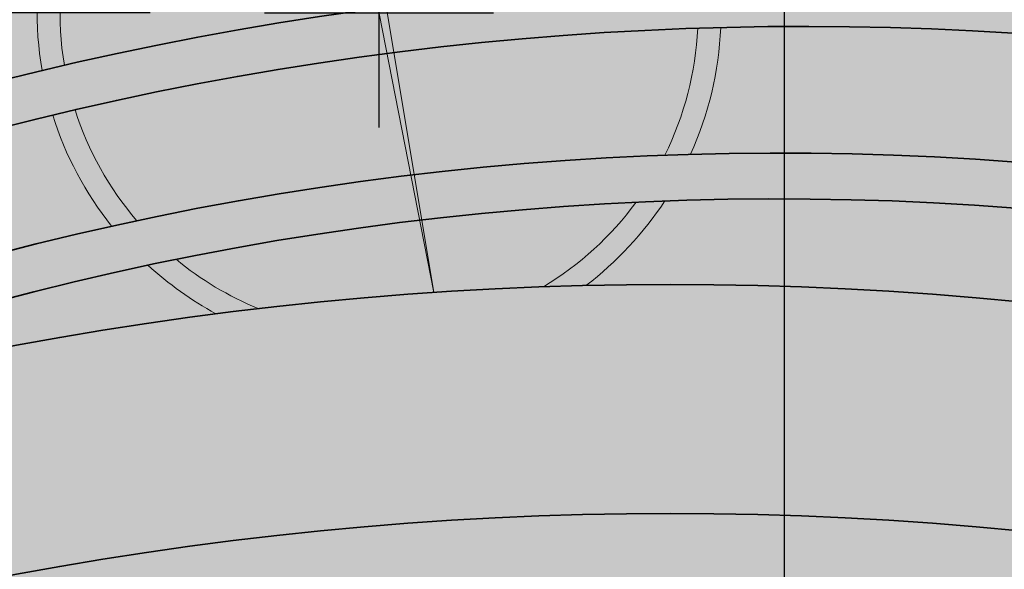
# Model space of a CAD drawing. Units: millimetres. Extents: x 130 to 1021, y 147 to 699.
# Tile 21 of 40: x 399 to 442, y 477 to 501. Entities that reach past the tile are written whole.
import ezdxf

# ---------------------------------------------------------------- set-up
doc = ezdxf.new("R2010")
doc.units = ezdxf.units.MM
doc.header["$MEASUREMENT"] = 0
for name, color, linetype, lineweight in [('A-ANNO-DIMS', 2, 'Continuous', 18), ('A-ELEV', 7, 'Continuous', 35), ('A-ELEV-PATT', 9, 'Continuous', 13), ('A-ELEV-RAIL', 6, 'Continuous', 18)]:
    doc.layers.add(name, color=color, linetype=linetype, lineweight=lineweight)
doc.styles.get("Standard").update_dxf_attribs({"font": 'arial.ttf'})
doc.dimstyles.get("Standard").update_dxf_attribs({"dimtxt": 20, "dimasz": 10, "dimexe": 10, "dimexo": 10, "dimgap": 5, "dimtad": 0, "dimtih": 1, "dimtoh": 1, "dimdec": 0, "dimzin": 0, "dimdsep": 46, "dimtxsty": 'Standard', "dimcen": 5, "dimadec": 0, "dimazin": 0, "dimtfac": 1, "dimtdec": 0, "dimtofl": 0, "dimtmove": 0, "dimatfit": 3, "dimfxl": 1, "dimtolj": 1, "dimtzin": 0, "dimarcsym": 0})

# ---------------------------------------------------------------- blocks, each defined once
blk = doc.blocks.new('*D11')
at = {"layer": 'A-ANNO-DIMS', "color": 0, "lineweight": -2, "transparency": 16777216}
for p, q in [((737.374, 648.699), (737.374, 149.739)), ((299.374, 566.947), (299.374, 149.739)), ((309.374, 159.739), (490.857, 159.739)), ((727.374, 159.739), (545.891, 159.739))]:
    blk.add_line(p, q, dxfattribs=at)
at = {"layer": 'A-ANNO-DIMS', "color": 0, "transparency": 16777216}
for points in [[(309.374, 161.406), (309.374, 158.073), (299.374, 159.739)], [(727.374, 161.406), (727.374, 158.073), (737.374, 159.739)]]:
    blk.add_solid(points, dxfattribs=at)
at = {"layer": 'Defpoints', "color": 0, "transparency": 16777216}
for p in [(737.374, 658.699), (299.374, 576.947), (737.374, 159.739)]:
    blk.add_point(p, dxfattribs=at)
at = {"layer": 'A-ANNO-DIMS', "color": 0, "transparency": 16777216, "insert": (518.374, 159.739), "char_height": 20, "attachment_point": 5}
blk.add_mtext('\\A1;438', dxfattribs=at)
blk = doc.blocks.new('*D12')
at = {"layer": 'A-ANNO-DIMS', "color": 0, "lineweight": -2, "transparency": 16777216}
for p, q in [((477.374, 661.947), (265.074, 661.947)), ((275.074, 651.947), (275.074, 438.205)), ((275.074, 194.039), (275.074, 407.782)), ((357.163, 184.039), (265.074, 184.039))]:
    blk.add_line(p, q, dxfattribs=at)
at = {"layer": 'A-ANNO-DIMS', "color": 0, "transparency": 16777216}
for points in [[(273.407, 651.947), (276.74, 651.947), (275.074, 661.947)], [(273.407, 194.039), (276.74, 194.039), (275.074, 184.039)]]:
    blk.add_solid(points, dxfattribs=at)
at = {"layer": 'Defpoints', "color": 0, "transparency": 16777216}
for p in [(275.074, 661.947), (487.374, 661.947), (367.163, 184.039)]:
    blk.add_point(p, dxfattribs=at)
at = {"layer": 'A-ANNO-DIMS', "color": 0, "transparency": 16777216, "insert": (275.074, 422.993), "char_height": 20, "attachment_point": 5}
blk.add_mtext('\\A1;477.9', dxfattribs=at)
blk = doc.blocks.new('*D15')
at = {"layer": 'A-ANNO-DIMS', "color": 0, "lineweight": -2, "transparency": 16777216}
for p, q in [((327.374, 579.884), (327.374, 696.247)), ((357.941, 411.947), (357.941, 696.247)), ((337.374, 686.247), (347.941, 686.247)), ((357.941, 686.247), (367.941, 686.247))]:
    blk.add_line(p, q, dxfattribs=at)
at = {"layer": 'A-ANNO-DIMS', "color": 0, "transparency": 16777216}
for points in [[(337.374, 687.914), (337.374, 684.581), (327.374, 686.247)], [(347.941, 687.914), (347.941, 684.581), (357.941, 686.247)]]:
    blk.add_solid(points, dxfattribs=at)
at = {"layer": 'Defpoints', "color": 0, "transparency": 16777216}
for p in [(357.941, 686.247), (327.374, 569.884), (357.941, 401.947)]:
    blk.add_point(p, dxfattribs=at)
at = {"layer": 'A-ANNO-DIMS', "color": 0, "transparency": 16777216, "insert": (406.679, 686.247), "char_height": 20, "attachment_point": 5}
blk.add_mtext('\\A1;30.57', dxfattribs=at)
blk = doc.blocks.new('*D16')
at = {"layer": 'A-ANNO-DIMS', "color": 0, "lineweight": -2, "transparency": 16777216}
for p, q in [((357.941, 411.947), (357.941, 696.247)), ((363.922, 579.884), (363.922, 696.247)), ((347.941, 686.247), (337.941, 686.247)), ((373.922, 686.247), (383.922, 686.247))]:
    blk.add_line(p, q, dxfattribs=at)
at = {"layer": 'A-ANNO-DIMS', "color": 0, "transparency": 16777216}
for points in [[(347.941, 687.914), (347.941, 684.581), (357.941, 686.247)], [(373.922, 687.914), (373.922, 684.581), (363.922, 686.247)]]:
    blk.add_solid(points, dxfattribs=at)
at = {"layer": 'Defpoints', "color": 0, "transparency": 16777216}
for p in [(363.922, 686.247), (363.922, 569.884), (357.941, 401.947)]:
    blk.add_point(p, dxfattribs=at)
at = {"layer": 'A-ANNO-DIMS', "color": 0, "transparency": 16777216, "insert": (420.737, 686.247), "char_height": 20, "attachment_point": 5}
blk.add_mtext('\\A1;5.981', dxfattribs=at)
blk = doc.blocks.new('*D17')
at = {"layer": 'A-ANNO-DIMS', "color": 0, "lineweight": -2, "transparency": 16777216}
for p, q in [((363.922, 579.884), (363.922, 696.247)), ((375.85, 490.216), (375.85, 696.247)), ((353.922, 686.247), (343.922, 686.247)), ((385.85, 686.247), (395.85, 686.247))]:
    blk.add_line(p, q, dxfattribs=at)
at = {"layer": 'A-ANNO-DIMS', "color": 0, "transparency": 16777216}
for points in [[(353.922, 687.914), (353.922, 684.581), (363.922, 686.247)], [(385.85, 687.914), (385.85, 684.581), (375.85, 686.247)]]:
    blk.add_solid(points, dxfattribs=at)
at = {"layer": 'Defpoints', "color": 0, "transparency": 16777216}
for p in [(375.85, 686.247), (363.922, 569.884), (375.85, 480.216)]:
    blk.add_point(p, dxfattribs=at)
at = {"layer": 'A-ANNO-DIMS', "color": 0, "transparency": 16777216, "insert": (441.444, 686.247), "char_height": 20, "attachment_point": 5}
blk.add_mtext('\\A1;11.928', dxfattribs=at)
blk = doc.blocks.new('*D18')
at = {"layer": 'A-ANNO-DIMS', "color": 0, "lineweight": -2, "transparency": 16777216}
for p, q in [((375.85, 490.216), (375.85, 696.247)), ((382.374, 388.947), (382.374, 696.247)), ((365.85, 686.247), (355.85, 686.247)), ((392.374, 686.247), (402.374, 686.247))]:
    blk.add_line(p, q, dxfattribs=at)
at = {"layer": 'A-ANNO-DIMS', "color": 0, "transparency": 16777216}
for points in [[(365.85, 687.914), (365.85, 684.581), (375.85, 686.247)], [(392.374, 687.914), (392.374, 684.581), (382.374, 686.247)]]:
    blk.add_solid(points, dxfattribs=at)
at = {"layer": 'Defpoints', "color": 0, "transparency": 16777216}
for p in [(382.374, 686.247), (375.85, 480.216), (382.374, 378.947)]:
    blk.add_point(p, dxfattribs=at)
at = {"layer": 'A-ANNO-DIMS', "color": 0, "transparency": 16777216, "insert": (441.132, 686.247), "char_height": 20, "attachment_point": 5}
blk.add_mtext('\\A1;6.524', dxfattribs=at)
blk = doc.blocks.new('*D19')
at = {"layer": 'A-ANNO-DIMS', "color": 0, "lineweight": -2, "transparency": 16777216}
for p, q in [((382.374, 388.947), (382.374, 696.247)), ((414.652, 510.881), (414.652, 696.247)), ((392.374, 686.247), (404.652, 686.247)), ((414.652, 686.247), (424.652, 686.247))]:
    blk.add_line(p, q, dxfattribs=at)
at = {"layer": 'A-ANNO-DIMS', "color": 0, "transparency": 16777216}
for points in [[(392.374, 687.914), (392.374, 684.581), (382.374, 686.247)], [(404.652, 687.914), (404.652, 684.581), (414.652, 686.247)]]:
    blk.add_solid(points, dxfattribs=at)
at = {"layer": 'Defpoints', "color": 0, "transparency": 16777216}
for p in [(414.652, 686.247), (414.652, 500.881), (382.374, 378.947)]:
    blk.add_point(p, dxfattribs=at)
at = {"layer": 'A-ANNO-DIMS', "color": 0, "transparency": 16777216, "insert": (463.411, 686.247), "char_height": 20, "attachment_point": 5}
blk.add_mtext('\\A1;32.28', dxfattribs=at)
blk = doc.blocks.new('*D20')
at = {"layer": 'A-ANNO-DIMS', "color": 0, "lineweight": -2, "transparency": 16777216}
for p, q in [((414.652, 510.881), (414.652, 696.247)), ((432.374, 388.947), (432.374, 696.247)), ((404.652, 686.247), (394.652, 686.247)), ((442.374, 686.247), (452.374, 686.247))]:
    blk.add_line(p, q, dxfattribs=at)
at = {"layer": 'A-ANNO-DIMS', "color": 0, "transparency": 16777216}
for points in [[(404.652, 687.914), (404.652, 684.581), (414.652, 686.247)], [(442.374, 687.914), (442.374, 684.581), (432.374, 686.247)]]:
    blk.add_solid(points, dxfattribs=at)
at = {"layer": 'Defpoints', "color": 0, "transparency": 16777216}
for p in [(432.374, 686.247), (414.652, 500.881), (432.374, 378.947)]:
    blk.add_point(p, dxfattribs=at)
at = {"layer": 'A-ANNO-DIMS', "color": 0, "transparency": 16777216, "insert": (490.075, 686.247), "char_height": 20, "attachment_point": 5}
blk.add_mtext('\\A1;17.72', dxfattribs=at)
blk = doc.blocks.new('*D21')
at = {"layer": 'A-ANNO-DIMS', "color": 0, "lineweight": -2, "transparency": 16777216}
for p, q in [((432.374, 388.947), (432.374, 696.247)), ((447.374, 656.947), (447.374, 696.247)), ((422.374, 686.247), (412.374, 686.247)), ((457.374, 686.247), (467.374, 686.247))]:
    blk.add_line(p, q, dxfattribs=at)
at = {"layer": 'A-ANNO-DIMS', "color": 0, "transparency": 16777216}
for points in [[(422.374, 687.914), (422.374, 684.581), (432.374, 686.247)], [(457.374, 687.914), (457.374, 684.581), (447.374, 686.247)]]:
    blk.add_solid(points, dxfattribs=at)
at = {"layer": 'Defpoints', "color": 0, "transparency": 16777216}
for p in [(447.374, 686.247), (447.374, 646.947), (432.374, 378.947)]:
    blk.add_point(p, dxfattribs=at)
at = {"layer": 'A-ANNO-DIMS', "color": 0, "transparency": 16777216, "insert": (485.832, 686.247), "char_height": 20, "attachment_point": 5}
blk.add_mtext('\\A1;15', dxfattribs=at)
blk = doc.blocks.new('*D22')
at = {"layer": 'A-ANNO-DIMS', "color": 0, "lineweight": -2, "transparency": 16777216}
for p, q in [((447.374, 656.947), (447.374, 696.247)), ((466.767, 403.947), (466.767, 696.247)), ((437.374, 686.247), (427.374, 686.247)), ((476.767, 686.247), (486.767, 686.247))]:
    blk.add_line(p, q, dxfattribs=at)
at = {"layer": 'A-ANNO-DIMS', "color": 0, "transparency": 16777216}
for points in [[(437.374, 687.914), (437.374, 684.581), (447.374, 686.247)], [(476.767, 687.914), (476.767, 684.581), (466.767, 686.247)]]:
    blk.add_solid(points, dxfattribs=at)
at = {"layer": 'Defpoints', "color": 0, "transparency": 16777216}
for p in [(466.767, 686.247), (447.374, 646.947), (466.767, 393.947)]:
    blk.add_point(p, dxfattribs=at)
at = {"layer": 'A-ANNO-DIMS', "color": 0, "transparency": 16777216, "insert": (532.34, 686.247), "char_height": 20, "attachment_point": 5}
blk.add_mtext('\\A1;19.393', dxfattribs=at)
blk = doc.blocks.new('*D43')
at = {"layer": 'A-ANNO-DIMS', "color": 0, "lineweight": -2, "transparency": 16777216}
for p, q in [((275.074, 510.881), (275.074, 520.881)), ((275.074, 520.881), (285.074, 520.881)), ((404.652, 500.881), (265.074, 500.881)), ((317.374, 480.95), (265.074, 480.95)), ((275.074, 470.95), (275.074, 460.95))]:
    blk.add_line(p, q, dxfattribs=at)
at = {"layer": 'A-ANNO-DIMS', "color": 0, "transparency": 16777216}
for points in [[(273.407, 510.881), (276.74, 510.881), (275.074, 500.881)], [(273.407, 470.95), (276.74, 470.95), (275.074, 480.95)]]:
    blk.add_solid(points, dxfattribs=at)
at = {"layer": 'Defpoints', "color": 0, "transparency": 16777216}
for p in [(275.074, 500.881), (414.652, 500.881), (327.374, 480.95)]:
    blk.add_point(p, dxfattribs=at)
at = {"layer": 'A-ANNO-DIMS', "color": 0, "transparency": 16777216, "insert": (322.877, 520.881), "char_height": 20, "attachment_point": 5}
blk.add_mtext('\\A1;19.93', dxfattribs=at)
blk = doc.blocks.new('*D62')
at = {"layer": 'A-ANNO-DIMS', "color": 0, "lineweight": -2, "transparency": 16777216}
for p, q in [((414.652, 495.881), (414.652, 505.881)), ((379.725, 501.926), (389.721, 501.627)), ((409.652, 500.881), (419.652, 500.881))]:
    blk.add_line(p, q, dxfattribs=at)
at = {"layer": 'A-ANNO-DIMS', "color": 0, "transparency": 16777216}
blk.add_solid([(389.771, 503.293), (389.671, 499.961), (399.716, 501.328)], dxfattribs=at)
at = {"layer": 'Defpoints', "color": 0, "transparency": 16777216}
for p in [(399.716, 501.328), (429.589, 500.434)]:
    blk.add_point(p, dxfattribs=at)
at = {"layer": 'A-ANNO-DIMS', "color": 0, "transparency": 16777216, "insert": (322.338, 501.926), "char_height": 20, "attachment_point": 5}
blk.add_mtext('\\A1;∅29.886', dxfattribs=at)
blk = doc.blocks.new('*D63')
at = {"layer": 'A-ANNO-DIMS', "color": 0, "lineweight": -2, "transparency": 16777216}
for p, q in [((414.652, 495.881), (414.652, 505.881)), ((380.753, 502.59), (390.74, 502.086)), ((409.652, 500.881), (419.652, 500.881))]:
    blk.add_line(p, q, dxfattribs=at)
at = {"layer": 'A-ANNO-DIMS', "color": 0, "transparency": 16777216}
blk.add_solid([(390.824, 503.751), (390.656, 500.422), (400.727, 501.583)], dxfattribs=at)
at = {"layer": 'Defpoints', "color": 0, "transparency": 16777216}
for p in [(400.727, 501.583), (428.578, 500.179)]:
    blk.add_point(p, dxfattribs=at)
at = {"layer": 'A-ANNO-DIMS', "color": 0, "transparency": 16777216, "insert": (323.365, 502.59), "char_height": 20, "attachment_point": 5}
blk.add_mtext('\\A1;∅27.886', dxfattribs=at)
blk = doc.blocks.new('*D65')
at = {"layer": 'A-ANNO-DIMS', "color": 0, "lineweight": -2, "transparency": 16777216}
for p, q in [((495.463, 509.127), (472.508, 423.108)), ((505.463, 509.127), (495.463, 509.127)), ((427.374, 248.979), (427.374, 258.979)), ((422.374, 253.979), (432.374, 253.979))]:
    blk.add_line(p, q, dxfattribs=at)
at = {"layer": 'A-ANNO-DIMS', "color": 0, "transparency": 16777216}
blk.add_solid([(470.898, 423.538), (474.118, 422.679), (469.93, 413.447)], dxfattribs=at)
at = {"layer": 'Defpoints', "color": 0, "transparency": 16777216}
for p in [(469.93, 413.447), (427.374, 253.979)]:
    blk.add_point(p, dxfattribs=at)
at = {"layer": 'A-ANNO-DIMS', "color": 0, "transparency": 16777216, "insert": (561.623, 509.127), "char_height": 20, "attachment_point": 5}
blk.add_mtext('\\A1;R165.05', dxfattribs=at)
blk = doc.blocks.new('*D66')
at = {"layer": 'A-ANNO-DIMS', "color": 0, "lineweight": -2, "transparency": 16777216}
for p, q in [((341.579, 557.194), (351.579, 557.194)), ((351.579, 557.194), (376.947, 478.135)), ((427.374, 315.978), (427.374, 325.978)), ((422.374, 320.978), (432.374, 320.978))]:
    blk.add_line(p, q, dxfattribs=at)
at = {"layer": 'A-ANNO-DIMS', "color": 0, "transparency": 16777216}
blk.add_solid([(378.534, 478.644), (375.36, 477.626), (380.002, 468.613)], dxfattribs=at)
at = {"layer": 'Defpoints', "color": 0, "transparency": 16777216}
for p in [(380.002, 468.613), (427.374, 320.978)]:
    blk.add_point(p, dxfattribs=at)
at = {"layer": 'A-ANNO-DIMS', "color": 0, "transparency": 16777216, "insert": (263.53, 557.194), "char_height": 20, "attachment_point": 5}
blk.add_mtext('\\A1;4X R155.05', dxfattribs=at)
blk = doc.blocks.new('*D67')
at = {"layer": 'A-ANNO-DIMS', "color": 0, "lineweight": -2, "transparency": 16777216}
for p, q in [((479.756, 492.431), (462.144, 412.223)), ((489.756, 492.431), (479.756, 492.431)), ((427.07, 247.496), (427.07, 257.496)), ((422.07, 252.496), (432.07, 252.496))]:
    blk.add_line(p, q, dxfattribs=at)
at = {"layer": 'A-ANNO-DIMS', "color": 0, "transparency": 16777216}
blk.add_solid([(460.516, 412.58), (463.772, 411.865), (459.999, 402.455)], dxfattribs=at)
at = {"layer": 'Defpoints', "color": 0, "transparency": 16777216}
for p in [(459.999, 402.455), (427.07, 252.496)]:
    blk.add_point(p, dxfattribs=at)
at = {"layer": 'A-ANNO-DIMS', "color": 0, "transparency": 16777216, "insert": (545.841, 492.431), "char_height": 20, "attachment_point": 5}
blk.add_mtext('\\A1;R153.53', dxfattribs=at)
blk = doc.blocks.new('*D68')
at = {"layer": 'A-ANNO-DIMS', "color": 0, "lineweight": -2, "transparency": 16777216}
for p, q in [((361.841, 579.756), (371.841, 579.756)), ((371.841, 579.756), (392.167, 506.693)), ((433.191, 354.23), (433.191, 364.23)), ((428.191, 359.23), (438.191, 359.23))]:
    blk.add_line(p, q, dxfattribs=at)
at = {"layer": 'A-ANNO-DIMS', "color": 0, "transparency": 16777216}
blk.add_solid([(393.773, 507.14), (390.561, 506.246), (394.847, 497.059)], dxfattribs=at)
at = {"layer": 'Defpoints', "color": 0, "transparency": 16777216}
for p in [(394.847, 497.059), (433.191, 359.23)]:
    blk.add_point(p, dxfattribs=at)
at = {"layer": 'A-ANNO-DIMS', "color": 0, "transparency": 16777216, "insert": (305.764, 579.756), "char_height": 20, "attachment_point": 5}
blk.add_mtext('\\A1;R143.06', dxfattribs=at)
blk = doc.blocks.new('*D69')
at = {"layer": 'A-ANNO-DIMS', "color": 0, "lineweight": -2, "transparency": 16777216}
for p, q in [((507.746, 572.261), (483.091, 501.813)), ((517.746, 572.261), (507.746, 572.261)), ((433.191, 354.23), (433.191, 364.23)), ((428.191, 359.23), (438.191, 359.23))]:
    blk.add_line(p, q, dxfattribs=at)
at = {"layer": 'A-ANNO-DIMS', "color": 0, "transparency": 16777216}
blk.add_solid([(481.518, 502.363), (484.664, 501.262), (479.788, 492.374)], dxfattribs=at)
at = {"layer": 'Defpoints', "color": 0, "transparency": 16777216}
for p in [(479.788, 492.374), (433.191, 359.23)]:
    blk.add_point(p, dxfattribs=at)
at = {"layer": 'A-ANNO-DIMS', "color": 0, "transparency": 16777216, "insert": (573.824, 572.261), "char_height": 20, "attachment_point": 5}
blk.add_mtext('\\A1;R141.06', dxfattribs=at)
blk = doc.blocks.new('*D70')
at = {"layer": 'A-ANNO-DIMS', "color": 0, "lineweight": -2, "transparency": 16777216}
for p, q in [((370.141, 588.4), (380.141, 588.4)), ((380.141, 588.4), (397.473, 517.008)), ((432.65, 367.109), (432.65, 377.109)), ((427.65, 372.109), (437.65, 372.109))]:
    blk.add_line(p, q, dxfattribs=at)
at = {"layer": 'A-ANNO-DIMS', "color": 0, "transparency": 16777216}
blk.add_solid([(399.093, 517.402), (395.854, 516.615), (399.832, 507.291)], dxfattribs=at)
at = {"layer": 'Defpoints', "color": 0, "transparency": 16777216}
for p in [(399.832, 507.291), (432.65, 372.109)]:
    blk.add_point(p, dxfattribs=at)
at = {"layer": 'A-ANNO-DIMS', "color": 0, "transparency": 16777216, "insert": (323.757, 588.4), "char_height": 20, "attachment_point": 5}
blk.add_mtext('\\A1;R139.1', dxfattribs=at)
blk = doc.blocks.new('*D71')
at = {"layer": 'A-ANNO-DIMS', "color": 0, "lineweight": -2, "transparency": 16777216}
for p, q in [((492.108, 581.609), (472.542, 512.666)), ((502.108, 581.609), (492.108, 581.609)), ((432.65, 367.109), (432.65, 377.109)), ((427.65, 372.109), (437.65, 372.109))]:
    blk.add_line(p, q, dxfattribs=at)
at = {"layer": 'A-ANNO-DIMS', "color": 0, "transparency": 16777216}
blk.add_solid([(470.938, 513.121), (474.145, 512.211), (469.812, 503.046)], dxfattribs=at)
at = {"layer": 'Defpoints', "color": 0, "transparency": 16777216}
for p in [(469.812, 503.046), (432.65, 372.109)]:
    blk.add_point(p, dxfattribs=at)
at = {"layer": 'A-ANNO-DIMS', "color": 0, "transparency": 16777216, "insert": (548.493, 581.609), "char_height": 20, "attachment_point": 5}
blk.add_mtext('\\A1;R136.1', dxfattribs=at)
blk = doc.blocks.new('*D72')
at = {"layer": 'A-ANNO-DIMS', "color": 0, "lineweight": -2, "transparency": 16777216}
for p, q in [((460.658, 573.64), (451.279, 503.49)), ((470.658, 573.64), (460.658, 573.64)), ((432.115, 355.142), (432.115, 365.142)), ((427.115, 360.142), (437.115, 360.142))]:
    blk.add_line(p, q, dxfattribs=at)
at = {"layer": 'A-ANNO-DIMS', "color": 0, "transparency": 16777216}
blk.add_solid([(449.628, 503.711), (452.931, 503.27), (449.954, 493.579)], dxfattribs=at)
at = {"layer": 'Defpoints', "color": 0, "transparency": 16777216}
for p in [(449.954, 493.579), (432.115, 360.142)]:
    blk.add_point(p, dxfattribs=at)
at = {"layer": 'A-ANNO-DIMS', "color": 0, "transparency": 16777216, "insert": (526.64, 573.64), "char_height": 20, "attachment_point": 5}
blk.add_mtext('\\A1;R134.62', dxfattribs=at)
blk = doc.blocks.new('*D73')
at = {"layer": 'A-ANNO-DIMS', "color": 0, "lineweight": -2, "transparency": 16777216}
for p, q in [((402.678, 571.448), (412.678, 571.448)), ((412.678, 571.448), (419.051, 502.166)), ((432.115, 355.142), (432.115, 365.142)), ((427.115, 360.142), (437.115, 360.142))]:
    blk.add_line(p, q, dxfattribs=at)
at = {"layer": 'A-ANNO-DIMS', "color": 0, "transparency": 16777216}
blk.add_solid([(420.711, 502.319), (417.391, 502.014), (419.967, 492.208)], dxfattribs=at)
at = {"layer": 'Defpoints', "color": 0, "transparency": 16777216}
for p in [(419.967, 492.208), (432.115, 360.142)]:
    blk.add_point(p, dxfattribs=at)
at = {"layer": 'A-ANNO-DIMS', "color": 0, "transparency": 16777216, "insert": (346.696, 571.448), "char_height": 20, "attachment_point": 5}
blk.add_mtext('\\A1;R132.62', dxfattribs=at)

msp = doc.modelspace()

# ---------------------------------------------------------------- hatches: boundary and pattern name
at = {"layer": 'A-ELEV-PATT'}
h = msp.add_hatch(color=256, dxfattribs=at)
h.dxf.hatch_style = 1
h.paths.add_polyline_path([(737.3738, 658.6988, 0.0135961), (632.4019, 661.9473), (607.3738, 661.9473), (487.3738, 661.9473), (487.3738, 649.9473), (607.3738, 649.9473), (632.3794, 649.9473, -0.0136841), (737.3738, 646.6784)])
h.paths.add_polyline_path([(732.3738, 643.9599, 0.0130529), (632.3738, 646.9473), (607.3738, 646.9473), (487.3738, 646.9473), (487.3738, 596.9473), (632.3738, 596.9473, -0.0130529), (732.3738, 593.9599)])
h.paths.add_polyline_path([(737.3738, 593.6732, 0.0137063), (632.3738, 596.9473), (487.3738, 596.9473), (487.3738, 586.9473), (632.355, 586.9473, -0.0137808), (737.3738, 583.6559)])
h.paths.add_polyline_path([(447.3738, 646.9473), (307.3738, 646.9473), (302.3738, 646.9473), (302.3738, 634.9473), (447.3738, 634.9473)])
h.paths.add_polyline_path([(447.3738, 631.9473), (307.3738, 631.9473), (307.3738, 586.9473), (447.3738, 586.9473)])
h.paths.add_polyline_path([(447.3738, 586.9473), (307.3738, 586.9473), (302.3738, 586.9473), (302.3738, 576.9473), (447.3738, 576.9473)])
h.paths.add_polyline_path([(447.3738, 573.9473), (367.3738, 573.9473), (367.3738, 539.9473), (447.3738, 539.9473)])
h.paths.add_polyline_path([(447.3738, 537.9473), (367.3738, 537.9473), (367.3738, 507.9473), (400.392, 507.4253, -0.001728), (401.3281, 507.6451, -0.5220025), (425.6117, 511.0391, -0.0391849), (447.3738, 510.4359), (447.3738, 510.7883)])
h.paths.add_polyline_path([(394.7238, 505.9473), (367.3738, 505.9473), (367.3738, 476.9473, -0.0146512), (375.8501, 480.2159), (376.1506, 499.2266, -0.0355419)])
h.paths.add_polyline_path([(632.3738, 583.9473), (552.3738, 583.9473), (552.3738, 550.9473), (632.3738, 550.9473)])
h.paths.add_polyline_path([(632.3738, 548.9473), (552.3738, 548.9473), (552.3738, 515.9473), (632.3738, 515.9473)])
h.paths.add_polyline_path([(632.3738, 513.9473), (552.3738, 513.9473), (552.3738, 476.9473), (632.3738, 476.9473)])
h.paths.add_polyline_path([(737.3738, 473.6903, 0.0136326), (632.3926, 476.9473), (552.3738, 476.9473), (487.3738, 476.9473), (487.3738, 466.9473), (632.3738, 466.9473, -0.0137063), (737.3738, 463.6732)])
h.paths.add_polyline_path([(732.3738, 460.9552, 0.0130741), (632.3681, 463.9473), (487.3738, 463.9473), (487.3738, 407.735, -0.0032286), (489.3544, 406.9473), (632.3926, 406.9473, -0.0129826), (732.3738, 403.9755)])
h.paths.add_polyline_path([(487.3738, 463.9473, 0.20133), (367.3738, 463.9473), (367.3738, 407.735, -0.1882031), (487.3738, 407.735)])
h.paths.add_polyline_path([(367.3738, 476.9473), (367.3738, 466.9473, -0.2013309), (487.3738, 466.9473), (487.3738, 476.9473, 0.20133)])
h.paths.add_polyline_path([(367.3738, 463.9473), (307.3738, 463.9473), (307.3738, 401.9473), (357.9413, 401.9473), (367.3738, 407.735)])
h.paths.add_polyline_path([(367.3738, 476.9473), (302.3738, 476.9473), (302.3738, 466.9473), (367.3738, 466.9473)])
h.paths.add_polyline_path([(632.8184, 366.9453), (552.3738, 366.9453), (552.3738, 393.9473), (632.8184, 393.9473)])
h.paths.add_polyline_path([(632.8184, 357.2114), (632.8184, 363.9453), (552.3738, 363.9453), (552.3738, 357.2114), (552.3738, 336.9453), (632.8184, 336.9453)])
h.paths.add_polyline_path([(632.8184, 333.9453), (552.3738, 333.9453), (552.3738, 306.9453), (632.8184, 306.9453)])
h.paths.add_polyline_path([(632.8184, 303.9453), (552.3738, 303.9453), (552.3738, 273.9473), (632.355, 273.9473, 0.0000608), (632.8184, 273.9491)])
h.paths.add_polyline_path([(737.3738, 403.6903, 0.0136326), (632.3926, 406.9473), (489.3544, 406.9473, 0.1915481), (367.3738, 407.735), (367.3738, 396.9473, -0.2013309), (487.3738, 396.9473), (632.3738, 396.9473, -0.0137063), (737.3738, 393.6732)])
h.paths.add_polyline_path([(357.9413, 401.9473), (307.3738, 401.9473), (307.3738, 391.9473), (357.9413, 391.9473)])
h.paths.add_polyline_path([(357.9413, 357.2114), (357.9413, 388.9473), (307.3738, 388.9473), (307.3738, 357.2114), (307.3738, 273.9473), (357.9413, 273.9473)])
h.paths.add_polyline_path([(732.3738, 263.93, -0.0130317), (632.3794, 260.9473), (466.7667, 260.9473), (466.7667, 240.9473), (469.8406, 236.978), (469.8406, 221.978), (472.9145, 218.0087), (472.9145, 213.9473), (607.3738, 213.9473), (732.3738, 213.9473)])
h.paths.add_polyline_path([(732.3738, 290.889), (722.479, 290.889), (722.479, 301.889), (732.3738, 301.889), (732.3738, 305.889), (722.479, 305.889), (722.479, 316.889), (732.3738, 316.889), (732.3738, 320.889), (722.479, 320.889), (722.479, 331.889), (732.3738, 331.889), (732.3738, 335.889), (722.479, 335.889), (722.479, 346.889), (732.3738, 346.889), (732.3738, 350.889), (722.479, 350.889), (722.479, 361.889), (732.3738, 361.889), (732.3738, 365.889), (722.479, 365.889), (722.479, 376.889), (732.3738, 376.889), (732.3738, 380.889), (722.479, 380.889), (722.479, 391.4848, 0.0005233), (718.479, 391.6843), (718.479, 380.889), (707.479, 380.889), (707.479, 392.1896, 0.0005231), (703.479, 392.3576), (703.479, 380.889), (692.479, 380.889), (692.479, 392.7765, 0.0005229), (688.479, 392.9131), (688.479, 380.889), (677.479, 380.889), (677.479, 393.2456, 0.0005228), (673.479, 393.3508), (673.479, 380.889), (662.479, 380.889), (662.479, 393.597, 0.0005227), (658.479, 393.6709), (658.479, 380.889), (647.479, 380.889), (647.479, 393.8308, 0.0005226), (643.479, 393.8732), (643.479, 380.889), (632.8184, 380.889), (632.8184, 376.889), (643.479, 376.889), (643.479, 365.889), (632.8184, 365.889), (632.8184, 361.889), (643.479, 361.889), (643.479, 350.889), (632.8184, 350.889), (632.8184, 346.889), (643.479, 346.889), (643.479, 335.889), (632.8184, 335.889), (632.8184, 331.889), (643.479, 331.889), (643.479, 320.889), (632.8184, 320.889), (632.8184, 316.889), (643.479, 316.889), (643.479, 305.889), (632.8184, 305.889), (632.8184, 301.889), (643.479, 301.889), (643.479, 290.889), (632.8184, 290.889), (632.8184, 286.889), (643.479, 286.889), (643.479, 274.0217, 0.0005246), (647.479, 274.0643), (647.479, 286.889), (658.479, 286.889), (658.479, 274.2248, 0.0005246), (662.479, 274.2989), (662.479, 286.889), (673.479, 286.889), (673.479, 274.546, 0.0005247), (677.479, 274.6516), (677.479, 286.889), (688.479, 286.889), (688.479, 274.9853, 0.0005248), (692.479, 275.1224), (692.479, 286.889), (703.479, 286.889), (703.479, 275.5429, 0.000525), (707.479, 275.7115), (707.479, 286.889), (718.479, 286.889), (718.479, 276.2187, 0.0005252), (722.479, 276.4189), (722.479, 286.889), (732.3738, 286.889)])
h.paths.add_polyline_path([(718.479, 290.889), (707.479, 290.889), (707.479, 301.889), (718.479, 301.889)], flags=16)
h.paths.add_polyline_path([(703.479, 290.889), (692.479, 290.889), (692.479, 301.889), (703.479, 301.889)], flags=16)
h.paths.add_polyline_path([(718.479, 305.889), (707.479, 305.889), (707.479, 316.889), (718.479, 316.889)], flags=16)
h.paths.add_polyline_path([(703.479, 305.889), (692.479, 305.889), (692.479, 316.889), (703.479, 316.889)], flags=16)
h.paths.add_polyline_path([(688.479, 290.889), (677.479, 290.889), (677.479, 301.889), (688.479, 301.889)], flags=16)
h.paths.add_polyline_path([(718.479, 320.889), (707.479, 320.889), (707.479, 331.889), (718.479, 331.889)], flags=16)
h.paths.add_polyline_path([(688.479, 305.889), (677.479, 305.889), (677.479, 316.889), (688.479, 316.889)], flags=16)
h.paths.add_polyline_path([(703.479, 320.889), (692.479, 320.889), (692.479, 331.889), (703.479, 331.889)], flags=16)
h.paths.add_polyline_path([(688.479, 320.889), (677.479, 320.889), (677.479, 331.889), (688.479, 331.889)], flags=16)
h.paths.add_polyline_path([(673.479, 290.889), (662.479, 290.889), (662.479, 301.889), (673.479, 301.889)], flags=16)
h.paths.add_polyline_path([(718.479, 335.889), (707.479, 335.889), (707.479, 346.889), (718.479, 346.889)], flags=16)
h.paths.add_polyline_path([(673.479, 305.889), (662.479, 305.889), (662.479, 316.889), (673.479, 316.889)], flags=16)
h.paths.add_polyline_path([(703.479, 335.889), (692.479, 335.889), (692.479, 346.889), (703.479, 346.889)], flags=16)
h.paths.add_polyline_path([(673.479, 320.889), (662.479, 320.889), (662.479, 331.889), (673.479, 331.889)], flags=16)
h.paths.add_polyline_path([(688.479, 335.889), (677.479, 335.889), (677.479, 346.889), (688.479, 346.889)], flags=16)
h.paths.add_polyline_path([(658.479, 290.889), (647.479, 290.889), (647.479, 301.889), (658.479, 301.889)], flags=16)
h.paths.add_polyline_path([(718.479, 350.889), (707.479, 350.889), (707.479, 361.889), (718.479, 361.889)], flags=16)
h.paths.add_polyline_path([(658.479, 305.889), (647.479, 305.889), (647.479, 316.889), (658.479, 316.889)], flags=16)
h.paths.add_polyline_path([(703.479, 350.889), (692.479, 350.889), (692.479, 361.889), (703.479, 361.889)], flags=16)
h.paths.add_polyline_path([(673.479, 335.889), (662.479, 335.889), (662.479, 346.889), (673.479, 346.889)], flags=16)
h.paths.add_polyline_path([(658.479, 320.889), (647.479, 320.889), (647.479, 331.889), (658.479, 331.889)], flags=16)
h.paths.add_polyline_path([(688.479, 350.889), (677.479, 350.889), (677.479, 361.889), (688.479, 361.889)], flags=16)
h.paths.add_polyline_path([(718.479, 365.889), (707.479, 365.889), (707.479, 376.889), (718.479, 376.889)], flags=16)
h.paths.add_polyline_path([(658.479, 335.889), (647.479, 335.889), (647.479, 346.889), (658.479, 346.889)], flags=16)
h.paths.add_polyline_path([(673.479, 350.889), (662.479, 350.889), (662.479, 361.889), (673.479, 361.889)], flags=16)
h.paths.add_polyline_path([(703.479, 365.889), (692.479, 365.889), (692.479, 376.889), (703.479, 376.889)], flags=16)
h.paths.add_polyline_path([(688.479, 365.889), (677.479, 365.889), (677.479, 376.889), (688.479, 376.889)], flags=16)
h.paths.add_polyline_path([(658.479, 350.889), (647.479, 350.889), (647.479, 361.889), (658.479, 361.889)], flags=16)
h.paths.add_polyline_path([(673.479, 365.889), (662.479, 365.889), (662.479, 376.889), (673.479, 376.889)], flags=16)
h.paths.add_polyline_path([(658.479, 365.889), (647.479, 365.889), (647.479, 376.889), (658.479, 376.889)], flags=16)
h.paths.add_polyline_path([(732.3738, 503.9786), (722.3392, 503.9786), (722.3392, 514.9786), (732.3738, 514.9786), (732.3738, 518.9786), (722.3392, 518.9786), (722.3392, 529.9786), (732.3738, 529.9786), (732.3738, 533.9786), (722.3392, 533.9786), (722.3392, 544.9786), (732.3738, 544.9786), (732.3738, 546.9473), (732.3738, 548.9786), (722.3392, 548.9786), (722.3392, 559.9786), (732.3738, 559.9786), (732.3738, 563.9786), (722.3392, 563.9786), (722.3392, 574.9786), (732.3738, 574.9786), (732.3738, 578.9786), (722.3392, 578.9786), (722.3392, 581.4789, 0.000526), (718.3392, 581.6791), (718.3392, 578.9786), (707.3392, 578.9786), (707.3392, 582.1863, 0.0005258), (703.3392, 582.355), (703.3392, 578.9786), (692.3392, 578.9786), (692.3392, 582.7752, 0.0005257), (688.3392, 582.9123), (688.3392, 578.9786), (677.3392, 578.9786), (677.3392, 583.2457, 0.0005255), (673.3392, 583.3512), (673.3392, 578.9786), (662.3392, 578.9786), (662.3392, 583.5978, 0.0005254), (658.3392, 583.6718), (658.3392, 578.9786), (647.3392, 578.9786), (647.3392, 583.8317, 0.0005254), (643.3392, 583.8741), (643.3392, 578.9786), (632.3738, 578.9786), (632.3738, 574.9786), (643.3392, 574.9786), (643.3392, 563.9786), (632.3738, 563.9786), (632.3738, 559.9786), (643.3392, 559.9786), (643.3392, 548.9786), (632.3738, 548.9786), (632.3738, 544.9786), (643.3392, 544.9786), (643.3392, 533.9786), (632.3738, 533.9786), (632.3738, 529.9786), (643.3392, 529.9786), (643.3392, 518.9786), (632.3738, 518.9786), (632.3738, 515.9473), (632.3738, 514.9786), (643.3392, 514.9786), (643.3392, 503.9786), (632.3738, 503.9786), (632.3738, 499.9786), (643.3392, 499.9786), (643.3392, 488.9786), (632.3738, 488.9786), (632.3738, 484.9786), (643.3392, 484.9786), (643.3392, 476.8751, -0.0005191), (647.3392, 476.8332), (647.3392, 484.9786), (658.3392, 484.9786), (658.3392, 476.6752, -0.0005192), (662.3392, 476.6022), (662.3392, 484.9786), (673.3392, 484.9786), (673.3392, 476.3585, -0.0005193), (677.3392, 476.2543), (677.3392, 484.9786), (688.3392, 484.9786), (688.3392, 475.9248, -0.0005194), (692.3392, 475.7894), (692.3392, 484.9786), (703.3392, 484.9786), (703.3392, 475.3741, -0.0005195), (707.3392, 475.2075), (707.3392, 484.9786), (718.3392, 484.9786), (718.3392, 474.7064, -0.0005197), (722.3392, 474.5086), (722.3392, 484.9786), (732.3738, 484.9786), (732.3738, 488.9786), (722.3392, 488.9786), (722.3392, 499.9786), (732.3738, 499.9786)])
h.paths.add_polyline_path([(718.3392, 503.9786), (707.3392, 503.9786), (707.3392, 514.9786), (718.3392, 514.9786)], flags=16)
h.paths.add_polyline_path([(718.3392, 499.9786), (718.3392, 488.9786), (707.3392, 488.9786), (707.3392, 499.9786)], flags=16)
h.paths.add_polyline_path([(718.3392, 518.9786), (707.3392, 518.9786), (707.3392, 529.9786), (718.3392, 529.9786)], flags=16)
h.paths.add_polyline_path([(703.3392, 503.9786), (692.3392, 503.9786), (692.3392, 514.9786), (703.3392, 514.9786)], flags=16)
h.paths.add_polyline_path([(703.3392, 499.9786), (703.3392, 488.9786), (692.3392, 488.9786), (692.3392, 499.9786)], flags=16)
h.paths.add_polyline_path([(703.3392, 518.9786), (692.3392, 518.9786), (692.3392, 529.9786), (703.3392, 529.9786)], flags=16)
h.paths.add_polyline_path([(718.3392, 533.9786), (707.3392, 533.9786), (707.3392, 544.9786), (718.3392, 544.9786)], flags=16)
h.paths.add_polyline_path([(688.3392, 503.9786), (677.3392, 503.9786), (677.3392, 514.9786), (688.3392, 514.9786)], flags=16)
h.paths.add_polyline_path([(688.3392, 499.9786), (688.3392, 488.9786), (677.3392, 488.9786), (677.3392, 499.9786)], flags=16)
h.paths.add_polyline_path([(703.3392, 533.9786), (692.3392, 533.9786), (692.3392, 544.9786), (703.3392, 544.9786)], flags=16)
h.paths.add_polyline_path([(688.3392, 518.9786), (677.3392, 518.9786), (677.3392, 529.9786), (688.3392, 529.9786)], flags=16)
h.paths.add_polyline_path([(688.3392, 533.9786), (677.3392, 533.9786), (677.3392, 544.9786), (688.3392, 544.9786)], flags=16)
h.paths.add_polyline_path([(718.3392, 548.9786), (707.3392, 548.9786), (707.3392, 559.9786), (718.3392, 559.9786)], flags=16)
h.paths.add_polyline_path([(673.3392, 503.9786), (662.3392, 503.9786), (662.3392, 514.9786), (673.3392, 514.9786)], flags=16)
h.paths.add_polyline_path([(673.3392, 499.9786), (673.3392, 488.9786), (662.3392, 488.9786), (662.3392, 499.9786)], flags=16)
h.paths.add_polyline_path([(703.3392, 548.9786), (692.3392, 548.9786), (692.3392, 559.9786), (703.3392, 559.9786)], flags=16)
h.paths.add_polyline_path([(673.3392, 518.9786), (662.3392, 518.9786), (662.3392, 529.9786), (673.3392, 529.9786)], flags=16)
h.paths.add_polyline_path([(688.3392, 548.9786), (677.3392, 548.9786), (677.3392, 559.9786), (688.3392, 559.9786)], flags=16)
h.paths.add_polyline_path([(673.3392, 533.9786), (662.3392, 533.9786), (662.3392, 544.9786), (673.3392, 544.9786)], flags=16)
h.paths.add_polyline_path([(718.3392, 563.9786), (707.3392, 563.9786), (707.3392, 574.9786), (718.3392, 574.9786)], flags=16)
h.paths.add_polyline_path([(658.3392, 503.9786), (647.3392, 503.9786), (647.3392, 514.9786), (658.3392, 514.9786)], flags=16)
h.paths.add_polyline_path([(658.3392, 499.9786), (658.3392, 488.9786), (647.3392, 488.9786), (647.3392, 499.9786)], flags=16)
h.paths.add_polyline_path([(703.3392, 563.9786), (692.3392, 563.9786), (692.3392, 574.9786), (703.3392, 574.9786)], flags=16)
h.paths.add_polyline_path([(658.3392, 518.9786), (647.3392, 518.9786), (647.3392, 529.9786), (658.3392, 529.9786)], flags=16)
h.paths.add_polyline_path([(673.3392, 548.9786), (662.3392, 548.9786), (662.3392, 559.9786), (673.3392, 559.9786)], flags=16)
h.paths.add_polyline_path([(688.3392, 563.9786), (677.3392, 563.9786), (677.3392, 574.9786), (688.3392, 574.9786)], flags=16)
h.paths.add_polyline_path([(658.3392, 533.9786), (647.3392, 533.9786), (647.3392, 544.9786), (658.3392, 544.9786)], flags=16)
h.paths.add_polyline_path([(673.3392, 563.9786), (662.3392, 563.9786), (662.3392, 574.9786), (673.3392, 574.9786)], flags=16)
h.paths.add_polyline_path([(658.3392, 548.9786), (647.3392, 548.9786), (647.3392, 559.9786), (658.3392, 559.9786)], flags=16)
h.paths.add_polyline_path([(658.3392, 563.9786), (647.3392, 563.9786), (647.3392, 574.9786), (658.3392, 574.9786)], flags=16)
h = msp.add_hatch(color=256, dxfattribs=at)
h.dxf.hatch_style = 1
h.paths.add_polyline_path([(447.3738, 576.9473), (302.3738, 576.9473), (302.3738, 573.9473), (447.3738, 573.9473)])
h.paths.add_polyline_path([(487.3738, 583.9473), (487.3738, 586.9473), (447.3738, 576.9473), (447.3738, 573.9473)])
h.paths.add_polyline_path([(632.355, 586.9473), (487.3738, 586.9473), (487.3738, 583.9473), (632.3738, 583.9473), (632.3738, 583.9472, -0.0138), (737.3738, 580.6507), (737.3738, 583.6559, 0.0137808)])
h.paths.add_polyline_path([(367.3738, 466.9473), (302.3738, 466.9473), (302.3738, 463.9473), (367.3738, 463.9473)])
h.paths.add_polyline_path([(487.3738, 463.9473), (487.3738, 466.9473, 0.2013309), (367.3738, 466.9473), (367.3738, 463.9473, -0.20133)])
h.paths.add_polyline_path([(632.3738, 466.9473), (487.3738, 466.9473), (487.3738, 463.9473), (632.3681, 463.9473, -0.0137285), (737.3738, 460.6681), (737.3738, 463.6732, 0.0137063)])
h.paths.add_polyline_path([(632.3738, 396.9473), (487.3738, 396.9473, 0.2013309), (367.3738, 396.9473), (367.3738, 393.9473, -0.2023717), (486.7667, 393.9473), (632.3681, 393.9473, -0.0137285), (737.3738, 390.6681), (737.3738, 393.6732, 0.0137063)])
h.paths.add_polyline_path([(357.9413, 391.9473), (307.3738, 391.9473), (307.3738, 388.9473), (357.9413, 388.9473)])
h.paths.add_polyline_path([(367.3738, 393.9473), (367.3738, 396.9473), (357.9413, 391.924), (357.9413, 388.9473), (358.058, 388.9473)])
h.paths.add_polyline_path([(737.3738, 264.2162), (737.3738, 267.2214, -0.0137063), (632.3738, 263.9473), (463.7667, 263.9473), (466.7667, 260.9473), (632.3794, 260.9473, 0.0136841)])
h.paths.add_polyline_path([(463.7667, 263.9473), (447.3738, 263.9473), (450.3738, 260.9473), (466.7667, 260.9473)])
h.paths.add_polyline_path([(447.3738, 263.9473), (432.3738, 263.9473), (432.3738, 260.9473), (450.3738, 260.9473)])
h.paths.add_polyline_path([(382.3738, 263.9473), (357.9413, 263.9473), (357.9413, 260.9473), (382.3738, 260.9473)])
h.paths.add_polyline_path([(357.9413, 263.9473), (307.3738, 263.9473), (307.3738, 260.9473), (357.9413, 260.9473)])
h = msp.add_hatch(color=256, dxfattribs=at)
h.paths.add_polyline_path([(424.2813, 510.9653, -0.0023948), (425.6117, 511.0391, 0.5220025), (401.3281, 507.6451, -0.0023948), (402.6278, 507.9389, -0.4837736)])
h.paths.add_polyline_path([(401.1963, 504.533, 0.002075), (400.0983, 504.2673, 0.0996756), (399.9219, 498.3708, -0.0017511), (400.8973, 498.6004, -0.1077432)])
h.paths.add_polyline_path([(401.3652, 496.6558, 0.0017772), (400.3891, 496.4261, 0.0927216), (402.9637, 491.5717, -0.0020893), (404.0631, 491.8108, -0.1004366)])
h.paths.add_polyline_path([(427.7205, 508.128, 0.002075), (426.5918, 508.0824, -0.1121628), (428.5313, 502.2169, -0.0017511), (429.5329, 502.2461, 0.1040877)])
h.paths.add_polyline_path([(429.5819, 500.2467, 0.0017772), (428.5796, 500.2174, -0.1038146), (427.1375, 494.6738, -0.0020893), (428.2619, 494.7107, 0.0960946)])
h.paths.add_polyline_path([(427.1388, 492.6724, 0.0023673), (425.8841, 492.6194, -0.0992667), (421.8309, 488.928, -0.0030044), (423.6933, 488.9834, 0.0850627)])
h.paths.add_polyline_path([(405.7805, 490.125, 0.0023673), (404.5509, 489.8698, 0.061248), (407.5193, 487.7506, -0.0030044), (409.3686, 487.9781, -0.0753981)])
h = msp.add_hatch(color=256, dxfattribs=at)
h.paths.add_polyline_path([(426.5918, 508.0824, 0.047204), (401.1963, 504.533, 0.1077432), (400.8973, 498.6004, -0.0488179), (428.5313, 502.2169, 0.1121628)])
h.paths.add_polyline_path([(424.2813, 510.9653, 0.4837736), (402.6278, 507.9389, -0.0393538)])
h.paths.add_polyline_path([(428.5796, 500.2174, 0.0487581), (401.3652, 496.6558, 0.1004366), (404.0631, 491.8108, -0.0432592), (427.1375, 494.6738, 0.1038146)])
h.paths.add_polyline_path([(425.8841, 492.6194, 0.0382424), (405.7805, 490.125, 0.0753981), (409.3686, 487.9781, -0.0201605), (421.8309, 488.928, 0.0992667)])
h = msp.add_hatch(color=256, dxfattribs=at)
h.paths.add_polyline_path([(375.8501, 480.2159, -0.0051389), (378.8667, 481.244), (378.8725, 481.6093, -0.2220519), (491.1023, 478.9257), (491.1023, 476.9473), (494.1023, 476.9473), (494.1023, 496.908, 0.2225165), (376.1506, 499.2266)])
h.paths.add_polyline_path([(379.1197, 497.2486, -0.2152592), (491.1023, 495.0271), (491.1023, 490.0474, 0.2040153), (379.0311, 491.6449)], flags=16)
h.paths.add_polyline_path([(491.1023, 487.8572), (491.1023, 481.1546, 0.1695534), (402.9637, 491.5717, -0.0927216), (400.3891, 496.4261, -0.1659296)], flags=16)
h = msp.add_hatch(color=256, dxfattribs=at)
h.paths.add_polyline_path([(399.9219, 498.3708, -0.0996756), (400.0983, 504.2673, 0.0406995), (379.1197, 497.2486), (379.0311, 491.6449, -0.0384084)])
h.paths.add_polyline_path([(402.9637, 491.5717, -0.0927216), (400.3891, 496.4261, 0.0399321), (378.9967, 489.4672), (378.9072, 483.8048, -0.0470483)])
h.paths.add_polyline_path([(404.5509, 489.8698, 0.0509798), (378.8725, 481.6093), (378.8667, 481.244, -0.0474823), (407.5193, 487.7506, -0.061248)])
h.paths.add_polyline_path([(447.3738, 491.8851, 0.0382282), (427.1388, 492.6724, -0.0850627), (423.6933, 488.9834, -0.0382916), (447.3738, 487.7318)])
h.paths.add_polyline_path([(447.3738, 499.578, 0.0315856), (429.5819, 500.2467, -0.0960946), (428.2619, 494.7107, -0.0355683), (447.3738, 493.8983)])
h.paths.add_polyline_path([(447.3738, 507.4186, 0.0361693), (427.7205, 508.128, -0.1040877), (429.5329, 502.2461, -0.0312283), (447.3738, 501.588)])

# ---------------------------------------------------------------- linework, layer by layer
at = {"layer": 'A-ELEV'}
for centre, radius, start, end in [((432.6505, 372.1087), 139.1086, 63.78413, 113.963624), ((432.6505, 372.1087), 136.1086, 64.567343, 113.15965), ((433.1906, 359.2304), 143.0624, 66.12141, 112.245303), ((433.1906, 359.2304), 141.0624, 65.761287, 112.593106), ((432.115, 360.1423), 134.6235, 64.013142, 113.246941), ((432.115, 360.1423), 132.6235, 63.591208, 113.669232), ((427.3738, 333.9781), 155.049, 67.23363, 112.76637), ((427.3738, 323.9788), 155.0484, 67.233534, 112.766466)]:
    msp.add_arc(centre, radius, start, end, dxfattribs=at)
at = {"layer": 'A-ELEV-RAIL'}
for p, q in [((412.7225, 514.6898), (417.0465, 488.6828)), ((417.0465, 488.6828), (411.9673, 514.563))]:
    msp.add_line(p, q, dxfattribs=at)
for radius, start, end in [(13.9429, 164.81619, 189.41422), (14.9429, 166.90225, 189.67102), (13.9429, 333.56429, 357.27193), (14.9429, 335.61091, 357.56674), (13.9429, 197.64019, 220.58163), (14.9429, 197.34537, 218.53501), (13.9429, 300.9868, 323.66277), (14.9429, 307.23065, 326.67877), (13.9429, 230.48315, 247.73048), (14.9429, 227.46715, 241.48664)]:
    msp.add_arc((414.6525, 500.8811), radius, start, end, dxfattribs=at)

# ---------------------------------------------------------------- dimensions: what is measured, and where the dimension line sits
at = {"layer": 'A-ANNO-DIMS'}
for base, p1, p2, override, picture, middle in [((357.9413, 686.2473), (327.3738, 569.884), (357.9413, 401.9473), {"dimdec": 2, "dimlfac": 1, "dimrnd": 0, "dimzin": 0, "dimdsep": 46, "dimlunit": 2}, '*D15', (406.6794, 686.2473)), ((363.922, 686.2473), (357.9413, 401.9473), (363.922, 569.884), {"dimdec": 3, "dimlfac": 1, "dimrnd": 0, "dimzin": 0, "dimdsep": 46, "dimlunit": 2}, '*D16', (420.7365, 686.2473)), ((375.8501, 686.2473), (363.922, 569.884), (375.8501, 480.2159), {"dimdec": 3, "dimlfac": 1, "dimrnd": 0, "dimzin": 0, "dimdsep": 46, "dimlunit": 2}, '*D17', (441.4435, 686.2473)), ((382.3738, 686.2473), (375.8501, 480.2159), (382.3738, 378.9473), {"dimdec": 3, "dimlfac": 1, "dimrnd": 0, "dimzin": 0, "dimdsep": 46, "dimlunit": 2}, '*D18', (441.1323, 686.2473)), ((414.6525, 686.2473), (382.3738, 378.9473), (414.6525, 500.8811), {"dimdec": 2, "dimlfac": 1, "dimrnd": 0, "dimzin": 0, "dimdsep": 46, "dimlunit": 2}, '*D19', (463.411, 686.2473)), ((432.3738, 686.2473), (414.6525, 500.8811), (432.3738, 378.9473), {"dimdec": 2, "dimlfac": 1, "dimrnd": 0, "dimzin": 0, "dimdsep": 46, "dimlunit": 2}, '*D20', (490.075, 686.2473)), ((447.3738, 686.2473), (432.3738, 378.9473), (447.3738, 646.9473), {"dimdec": 0, "dimlfac": 1, "dimrnd": 0, "dimzin": 0, "dimdsep": 46, "dimlunit": 2}, '*D21', (485.8322, 686.2473)), ((466.7667, 686.2473), (447.3738, 646.9473), (466.7667, 393.9473), {"dimdec": 3, "dimlfac": 1, "dimrnd": 0, "dimzin": 0, "dimdsep": 46, "dimlunit": 2}, '*D22', (532.3397, 686.2473)), ((737.3738, 159.7395), (299.3738, 576.9473), (737.3738, 658.6988), {"dimdec": 0, "dimlfac": 1, "dimrnd": 0, "dimzin": 0, "dimdsep": 46, "dimlunit": 2}, '*D11', (518.3738, 159.7395))]:
    dim = msp.add_linear_dim(base=base, p1=p1, p2=p2, dimstyle='Standard', override=override, dxfattribs=at)
    dim.commit()
    dim.dimension.update_dxf_attribs({"geometry": picture, "text_midpoint": middle})
for base, p1, p2, override, picture, middle in [((275.0738, 661.9473), (367.163, 184.0395), (487.3738, 661.9473), {"dimdec": 1, "dimlfac": 1, "dimrnd": 0, "dimzin": 0, "dimdsep": 46, "dimlunit": 2}, '*D12', (275.0738, 422.9934)), ((275.0738, 500.8811), (327.3738, 480.95), (414.6525, 500.8811), {"dimdec": 2, "dimlfac": 1, "dimrnd": 0, "dimzin": 0, "dimdsep": 46, "dimlunit": 2}, '*D43', (322.8773, 520.8811))]:
    dim = msp.add_linear_dim(base=base, p1=p1, p2=p2, angle=90, dimstyle='Standard', override=override, dxfattribs=at)
    dim.commit()
    dim.dimension.update_dxf_attribs({"geometry": picture, "text_midpoint": middle})
for center, mpoint, override, picture, middle in [((432.6505, 372.1087), (399.8323, 507.2907), {"dimdec": 1, "dimlfac": 1, "dimrnd": 0, "dimzin": 0, "dimdsep": 46, "dimlunit": 2}, '*D70', (323.7567, 588.3999)), ((432.6505, 372.1087), (469.8116, 503.0461), {"dimdec": 1, "dimlfac": 1, "dimrnd": 0, "dimzin": 0, "dimdsep": 46, "dimlunit": 2}, '*D71', (548.493, 581.6085)), ((433.1906, 359.2304), (394.8473, 497.0587), {"dimdec": 2, "dimlfac": 1, "dimrnd": 0, "dimzin": 0, "dimdsep": 46, "dimlunit": 2}, '*D68', (305.7636, 579.7557)), ((432.115, 360.1423), (449.9544, 493.5786), {"dimdec": 2, "dimlfac": 1, "dimrnd": 0, "dimzin": 0, "dimdsep": 46, "dimlunit": 2}, '*D72', (526.6403, 573.6404)), ((433.1906, 359.2304), (479.788, 492.3743), {"dimdec": 2, "dimlfac": 1, "dimrnd": 0, "dimzin": 0, "dimdsep": 46, "dimlunit": 2}, '*D69', (573.8242, 572.2606)), ((432.115, 360.1423), (419.967, 492.2083), {"dimdec": 2, "dimlfac": 1, "dimrnd": 0, "dimzin": 0, "dimdsep": 46, "dimlunit": 2}, '*D73', (346.696, 571.4479)), ((427.3738, 253.9788), (469.9297, 413.4465), {"dimdec": 2, "dimlfac": 1, "dimrnd": 0, "dimzin": 0, "dimdsep": 46, "dimlunit": 2}, '*D65', (561.6228, 509.1272)), ((427.0702, 252.4956), (459.999, 402.4554), {"dimdec": 2, "dimlfac": 1, "dimrnd": 0, "dimzin": 0, "dimdsep": 46, "dimlunit": 2}, '*D67', (545.8408, 492.4313))]:
    dim = msp.add_radius_dim(center=center, mpoint=mpoint, dimstyle='Standard', override=override, dxfattribs=at)
    dim.commit()
    dim.dimension.update_dxf_attribs({"geometry": picture, "text_midpoint": middle, "dimtype": 164})
dim = msp.add_radius_dim(center=(427.3738, 320.9781), mpoint=(380.0022, 468.6132), text='4X <>', dimstyle='Standard', override={"dimdec": 2, "dimlfac": 1, "dimrnd": 0, "dimzin": 0, "dimdsep": 46, "dimlunit": 2}, dxfattribs=at)
dim.commit()
dim.dimension.update_dxf_attribs({"geometry": '*D66', "text_midpoint": (263.5301, 557.1943), "dimtype": 164})
for p1, p2, picture, middle in [((428.5777, 500.1791), (400.7272, 501.583), '*D63', (380.7526, 502.5898)), ((429.5887, 500.4341), (399.7162, 501.328), '*D62', (379.7252, 501.9262))]:
    dim = msp.add_diameter_dim_2p(p1=p1, p2=p2, dimstyle='Standard', override={"dimdec": 3, "dimlfac": 1, "dimrnd": 0, "dimzin": 0, "dimdsep": 46, "dimlunit": 2}, dxfattribs=at)
    dim.commit()
    dim.dimension.update_dxf_attribs({"geometry": picture, "text_midpoint": middle, "dimtype": 163})

doc.saveas('drawing.dxf')
